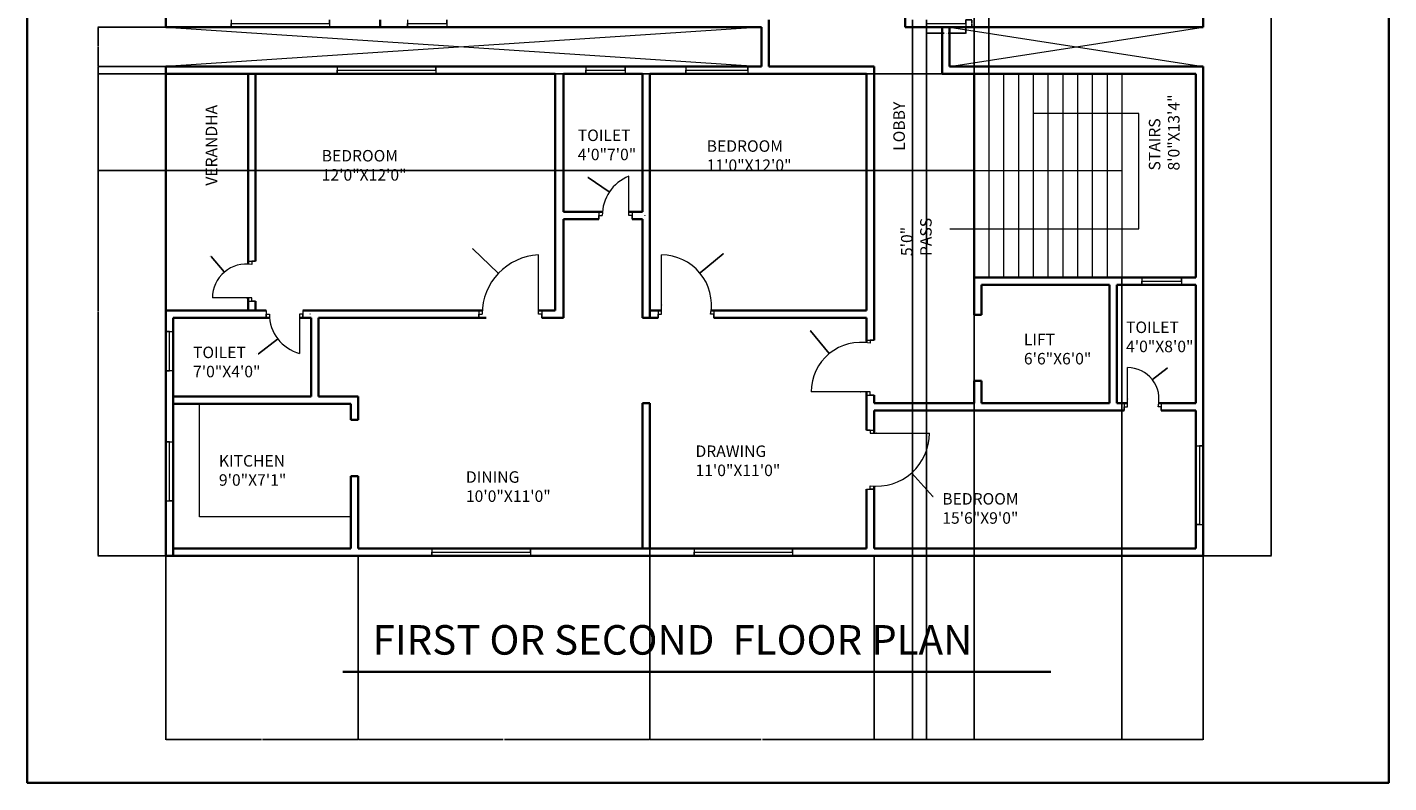
# Model space of a CAD drawing. Units: inches. Extents: x 6393 to 7221, y 6416 to 7347.
# Tile 1 of 3: x 6393 to 7221, y 6416 to 6876. Entities that reach past the tile are written whole.
import ezdxf

# ---------------------------------------------------------------- set-up
doc = ezdxf.new("R2010")
doc.units = ezdxf.units.IN
for name, color, linetype, lineweight in [('A-ANNO-DIMS', 2, 'Continuous', 18), ('A-ANNO-TEXT', 7, 'Continuous', 35), ('A-ANNO-TTLB', 7, 'Continuous', 35), ('A-AREA-IDEN', 7, 'Continuous', 18), ('A-DOOR', 3, 'Continuous', 18), ('A-FLOR-FIXT', 8, 'Continuous', 18), ('A-FLOR-OPEN', 8, 'Continuous', 13), ('A-FLOR-STRS', 7, 'Continuous', 18), ('A-GLAZ', 4, 'Continuous', 18), ('A-WALL', 7, 'Continuous', 35)]:
    doc.layers.add(name, color=color, linetype=linetype, lineweight=lineweight)
doc.styles.get("Standard").update_dxf_attribs({"font": 'arial.ttf'})
doc.dimstyles.get("Standard").update_dxf_attribs({"dimtxt": 0.18, "dimasz": 0.18, "dimexe": 0.18, "dimexo": 0.0625, "dimgap": 0.09, "dimtad": 0, "dimtih": 1, "dimtoh": 1, "dimdec": 4, "dimzin": 0, "dimdsep": 46, "dimtxsty": 'Standard', "dimcen": 0.09, "dimadec": 0, "dimazin": 0, "dimtfac": 1, "dimtdec": 4, "dimtofl": 0, "dimtmove": 0, "dimatfit": 3, "dimfxl": 1, "dimtolj": 1, "dimtzin": 0, "dimarcsym": 0})

# ---------------------------------------------------------------- blocks, each defined once
blk = doc.blocks.new('WIN-60IN')
for p, q in [((0, 60), (4.5, 60)), ((4.5, 60), (2.25, 60)), ((2.25, 60), (2.25, 0)), ((2.25, 0), (0, 0)), ((0, 0), (4.5, 0))]:
    blk.add_line(p, q)
blk = doc.blocks.new('WIN-24IN')
for p, q in [((0, 4.5), (0, 0)), ((0, 0), (0, 2.25)), ((0, 2.25), (24, 2.25)), ((24, 2.25), (24, 4.5)), ((24, 4.5), (24, 0))]:
    blk.add_line(p, q)
blk = doc.blocks.new('WIN-48IN')
for p, q in [((0, 4.5), (0, 0)), ((0, 0), (0, 2.25)), ((0, 2.25), (48, 2.25)), ((48, 2.25), (48, 4.5)), ((48, 4.5), (48, 0))]:
    blk.add_line(p, q)
blk = doc.blocks.new('*D7')
at = {"layer": 'A-ANNO-DIMS', "color": 0, "lineweight": -2, "transparency": 16777216}
for p, q in [((6939.9, 6876.26), (6939.9, 6872.55)), ((6940.08, 6872.73), (6950.67, 6872.73)), ((6963.72, 6872.73), (6953.14, 6872.73)), ((6963.9, 6876.26), (6963.9, 6872.55))]:
    blk.add_line(p, q, dxfattribs=at)
at = {"layer": 'A-ANNO-DIMS', "color": 0, "transparency": 16777216}
for points in [[(6940.08, 6872.76), (6940.08, 6872.7), (6939.9, 6872.73)], [(6963.72, 6872.76), (6963.72, 6872.7), (6963.9, 6872.73)]]:
    blk.add_solid(points, dxfattribs=at)
at = {"layer": 'Defpoints', "color": 0, "transparency": 16777216}
for p in [(6939.9, 6876.33), (6963.9, 6876.33), (6963.9, 6872.73)]:
    blk.add_point(p, dxfattribs=at)
at = {"layer": 'A-ANNO-DIMS', "color": 0, "transparency": 16777216, "insert": (6951.9, 6872.73), "char_height": 0.18, "attachment_point": 5}
blk.add_mtext('\\A1;WINDOW B 24 TYP.', dxfattribs=at)
blk = doc.blocks.new('*D8')
at = {"layer": 'A-ANNO-DIMS', "color": 0, "lineweight": -2, "transparency": 16777216}
for p, q in [((6963.97, 6880.83), (6967.68, 6880.83)), ((6967.5, 6880.65), (6967.5, 6878.76)), ((6963.97, 6876.33), (6967.68, 6876.33)), ((6967.5, 6876.51), (6967.5, 6878.4))]:
    blk.add_line(p, q, dxfattribs=at)
at = {"layer": 'A-ANNO-DIMS', "color": 0, "transparency": 16777216}
for points in [[(6967.47, 6880.65), (6967.53, 6880.65), (6967.5, 6880.83)], [(6967.47, 6876.51), (6967.53, 6876.51), (6967.5, 6876.33)]]:
    blk.add_solid(points, dxfattribs=at)
at = {"layer": 'Defpoints', "color": 0, "transparency": 16777216}
for p in [(6963.9, 6880.83), (6967.5, 6880.83), (6963.9, 6876.33)]:
    blk.add_point(p, dxfattribs=at)
at = {"layer": 'A-ANNO-DIMS', "color": 0, "transparency": 16777216, "insert": (6967.5, 6878.58), "char_height": 0.18, "attachment_point": 5}
blk.add_mtext('\\A1;5 TYP.', dxfattribs=at)
blk = doc.blocks.new('*D14')
at = {"layer": 'A-ANNO-DIMS', "color": 0, "lineweight": -2, "transparency": 16777216}
for p, q in [((7108.59, 7305.82), (7149.96, 7305.82)), ((7149.78, 7305.64), (7149.78, 6930.26)), ((7149.78, 6554.51), (7149.78, 6929.89)), ((7108.49, 6554.33), (7149.96, 6554.33))]:
    blk.add_line(p, q, dxfattribs=at)
at = {"layer": 'A-ANNO-DIMS', "color": 0, "transparency": 16777216}
for points in [[(7149.75, 7305.64), (7149.81, 7305.64), (7149.78, 7305.82)], [(7149.75, 6554.51), (7149.81, 6554.51), (7149.78, 6554.33)]]:
    blk.add_solid(points, dxfattribs=at)
at = {"layer": 'Defpoints', "color": 0, "transparency": 16777216}
for p in [(7108.53, 7305.82), (7149.78, 7305.82), (7108.43, 6554.33)]:
    blk.add_point(p, dxfattribs=at)
at = {"layer": 'A-ANNO-DIMS', "color": 0, "transparency": 16777216, "insert": (7149.78, 6930.07), "char_height": 0.18, "attachment_point": 5}
blk.add_mtext('\\A1;751.5', dxfattribs=at)
blk = doc.blocks.new('*D15')
at = {"layer": 'A-ANNO-DIMS', "color": 0, "lineweight": -2, "transparency": 16777216}
for p, q in [((6476.86, 6852.33), (6435.5, 6852.33)), ((6435.68, 6852.15), (6435.68, 6703.51)), ((6435.68, 6554.51), (6435.68, 6703.14)), ((6476.86, 6554.33), (6435.5, 6554.33))]:
    blk.add_line(p, q, dxfattribs=at)
at = {"layer": 'A-ANNO-DIMS', "color": 0, "transparency": 16777216}
for points in [[(6435.65, 6852.15), (6435.71, 6852.15), (6435.68, 6852.33)], [(6435.65, 6554.51), (6435.71, 6554.51), (6435.68, 6554.33)]]:
    blk.add_solid(points, dxfattribs=at)
at = {"layer": 'Defpoints', "color": 0, "transparency": 16777216}
for p in [(6435.68, 6852.33), (6476.93, 6852.33), (6476.93, 6554.33)]:
    blk.add_point(p, dxfattribs=at)
at = {"layer": 'A-ANNO-DIMS', "color": 0, "transparency": 16777216, "insert": (6435.68, 6703.33), "char_height": 0.18, "attachment_point": 5}
blk.add_mtext('\\A1;298', dxfattribs=at)
blk = doc.blocks.new('*D16')
at = {"layer": 'A-ANNO-DIMS', "color": 0, "lineweight": -2, "transparency": 16777216}
for p, q in [((6476.86, 6876.33), (6435.5, 6876.33)), ((6435.68, 6876.15), (6435.68, 6864.51)), ((6435.68, 6852.51), (6435.68, 6864.15)), ((6476.86, 6852.33), (6435.5, 6852.33))]:
    blk.add_line(p, q, dxfattribs=at)
at = {"layer": 'A-ANNO-DIMS', "color": 0, "transparency": 16777216}
for points in [[(6435.65, 6876.15), (6435.71, 6876.15), (6435.68, 6876.33)], [(6435.65, 6852.51), (6435.71, 6852.51), (6435.68, 6852.33)]]:
    blk.add_solid(points, dxfattribs=at)
at = {"layer": 'Defpoints', "color": 0, "transparency": 16777216}
for p in [(6435.68, 6876.33), (6476.93, 6876.33), (6476.93, 6852.33)]:
    blk.add_point(p, dxfattribs=at)
at = {"layer": 'A-ANNO-DIMS', "color": 0, "transparency": 16777216, "insert": (6435.68, 6864.33), "char_height": 0.18, "attachment_point": 5}
blk.add_mtext('\\A1;24', dxfattribs=at)
blk = doc.blocks.new('*D22')
at = {"layer": 'A-ANNO-DIMS', "color": 0, "lineweight": -2, "transparency": 16777216}
for p, q in [((6476.93, 6554.26), (6476.93, 6442.29)), ((6593.93, 6554.26), (6593.93, 6442.29)), ((6477.11, 6442.47), (6535.15, 6442.47)), ((6593.75, 6442.47), (6535.71, 6442.47))]:
    blk.add_line(p, q, dxfattribs=at)
at = {"layer": 'A-ANNO-DIMS', "color": 0, "transparency": 16777216}
for points in [[(6477.11, 6442.5), (6477.11, 6442.44), (6476.93, 6442.47)], [(6593.75, 6442.5), (6593.75, 6442.44), (6593.93, 6442.47)]]:
    blk.add_solid(points, dxfattribs=at)
at = {"layer": 'Defpoints', "color": 0, "transparency": 16777216}
for p in [(6476.93, 6554.33), (6593.93, 6554.33), (6593.93, 6442.47)]:
    blk.add_point(p, dxfattribs=at)
at = {"layer": 'A-ANNO-DIMS', "color": 0, "transparency": 16777216, "insert": (6535.43, 6442.47), "char_height": 0.18, "attachment_point": 5}
blk.add_mtext('\\A1;117', dxfattribs=at)
blk = doc.blocks.new('*D23')
at = {"layer": 'A-ANNO-DIMS', "color": 0, "lineweight": -2, "transparency": 16777216}
for p, q in [((6771.53, 6558.76), (6771.53, 6442.29)), ((6593.93, 6554.26), (6593.93, 6442.29)), ((6594.11, 6442.47), (6682.34, 6442.47)), ((6771.35, 6442.47), (6683.12, 6442.47))]:
    blk.add_line(p, q, dxfattribs=at)
at = {"layer": 'A-ANNO-DIMS', "color": 0, "transparency": 16777216}
for points in [[(6594.11, 6442.5), (6594.11, 6442.44), (6593.93, 6442.47)], [(6771.35, 6442.5), (6771.35, 6442.44), (6771.53, 6442.47)]]:
    blk.add_solid(points, dxfattribs=at)
at = {"layer": 'Defpoints', "color": 0, "transparency": 16777216}
for p in [(6771.53, 6558.83), (6593.93, 6554.33), (6771.53, 6442.47)]:
    blk.add_point(p, dxfattribs=at)
at = {"layer": 'A-ANNO-DIMS', "color": 0, "transparency": 16777216, "insert": (6682.73, 6442.47), "char_height": 0.18, "attachment_point": 5}
blk.add_mtext('\\A1;177.6', dxfattribs=at)
blk = doc.blocks.new('*D24')
at = {"layer": 'A-ANNO-DIMS', "color": 0, "lineweight": -2, "transparency": 16777216}
for p, q in [((6771.53, 6558.76), (6771.53, 6442.29)), ((6908.03, 6554.26), (6908.03, 6442.29)), ((6771.71, 6442.47), (6839.4, 6442.47)), ((6907.85, 6442.47), (6840.17, 6442.47))]:
    blk.add_line(p, q, dxfattribs=at)
at = {"layer": 'A-ANNO-DIMS', "color": 0, "transparency": 16777216}
for points in [[(6771.71, 6442.5), (6771.71, 6442.44), (6771.53, 6442.47)], [(6907.85, 6442.5), (6907.85, 6442.44), (6908.03, 6442.47)]]:
    blk.add_solid(points, dxfattribs=at)
at = {"layer": 'Defpoints', "color": 0, "transparency": 16777216}
for p in [(6771.53, 6558.83), (6908.03, 6554.33), (6908.03, 6442.47)]:
    blk.add_point(p, dxfattribs=at)
at = {"layer": 'A-ANNO-DIMS', "color": 0, "transparency": 16777216, "insert": (6839.78, 6442.47), "char_height": 0.18, "attachment_point": 5}
blk.add_mtext('\\A1;136.5', dxfattribs=at)
blk = doc.blocks.new('*D25')
at = {"layer": 'A-ANNO-DIMS', "color": 0, "lineweight": -2, "transparency": 16777216}
for p, q in [((6908.03, 6554.26), (6908.03, 6442.29)), ((7108.43, 6554.26), (7108.43, 6442.29)), ((6908.21, 6442.47), (7007.84, 6442.47)), ((7108.25, 6442.47), (7008.62, 6442.47))]:
    blk.add_line(p, q, dxfattribs=at)
at = {"layer": 'A-ANNO-DIMS', "color": 0, "transparency": 16777216}
for points in [[(6908.21, 6442.5), (6908.21, 6442.44), (6908.03, 6442.47)], [(7108.25, 6442.5), (7108.25, 6442.44), (7108.43, 6442.47)]]:
    blk.add_solid(points, dxfattribs=at)
at = {"layer": 'Defpoints', "color": 0, "transparency": 16777216}
for p in [(6908.03, 6554.33), (7108.43, 6554.33), (7108.43, 6442.47)]:
    blk.add_point(p, dxfattribs=at)
at = {"layer": 'A-ANNO-DIMS', "color": 0, "transparency": 16777216, "insert": (7008.23, 6442.47), "char_height": 0.18, "attachment_point": 5}
blk.add_mtext('\\A1;200.4', dxfattribs=at)
blk = doc.blocks.new('*D29')
at = {"layer": 'A-ANNO-DIMS', "color": 0, "lineweight": -2, "transparency": 16777216}
for p, q in [((6968.93, 6847.89), (6968.93, 7347.25)), ((6969.11, 7347.07), (6973.28, 7347.07)), ((6977.75, 7347.07), (6973.58, 7347.07)), ((6977.93, 6847.89), (6977.93, 7347.25))]:
    blk.add_line(p, q, dxfattribs=at)
at = {"layer": 'A-ANNO-DIMS', "color": 0, "transparency": 16777216}
for points in [[(6969.11, 7347.1), (6969.11, 7347.04), (6968.93, 7347.07)], [(6977.75, 7347.1), (6977.75, 7347.04), (6977.93, 7347.07)]]:
    blk.add_solid(points, dxfattribs=at)
at = {"layer": 'Defpoints', "color": 0, "transparency": 16777216}
for p in [(6977.93, 7347.07), (6968.93, 6847.83), (6977.93, 6847.83)]:
    blk.add_point(p, dxfattribs=at)
at = {"layer": 'A-ANNO-DIMS', "color": 0, "transparency": 16777216, "insert": (6973.43, 7347.07), "char_height": 0.18, "attachment_point": 5}
blk.add_mtext('\\A1;9', dxfattribs=at)
blk = doc.blocks.new('*D30')
at = {"layer": 'A-ANNO-DIMS', "color": 0, "lineweight": -2, "transparency": 16777216}
for p, q in [((6968.93, 6723.75), (6968.93, 6442.29)), ((7058.93, 6723.75), (7058.93, 6442.29)), ((6969.11, 6442.47), (7013.71, 6442.47)), ((7058.75, 6442.47), (7014.15, 6442.47))]:
    blk.add_line(p, q, dxfattribs=at)
at = {"layer": 'A-ANNO-DIMS', "color": 0, "transparency": 16777216}
for points in [[(6969.11, 6442.5), (6969.11, 6442.44), (6968.93, 6442.47)], [(7058.75, 6442.5), (7058.75, 6442.44), (7058.93, 6442.47)]]:
    blk.add_solid(points, dxfattribs=at)
at = {"layer": 'Defpoints', "color": 0, "transparency": 16777216}
for p in [(6968.93, 6723.82), (7058.93, 6723.82), (7058.93, 6442.47)]:
    blk.add_point(p, dxfattribs=at)
at = {"layer": 'A-ANNO-DIMS', "color": 0, "transparency": 16777216, "insert": (7013.93, 6442.47), "char_height": 0.18, "attachment_point": 5}
blk.add_mtext('\\A1;90', dxfattribs=at)
blk = doc.blocks.new('*D31')
at = {"layer": 'A-ANNO-DIMS', "color": 0, "lineweight": -2, "transparency": 16777216}
for p, q in [((6968.86, 6847.83), (6435.5, 6847.83)), ((6435.68, 6847.65), (6435.68, 6818.65)), ((6435.68, 6789.28), (6435.68, 6818.28)), ((6968.86, 6789.1), (6435.5, 6789.1))]:
    blk.add_line(p, q, dxfattribs=at)
at = {"layer": 'A-ANNO-DIMS', "color": 0, "transparency": 16777216}
for points in [[(6435.65, 6847.65), (6435.71, 6847.65), (6435.68, 6847.83)], [(6435.65, 6789.28), (6435.71, 6789.28), (6435.68, 6789.1)]]:
    blk.add_solid(points, dxfattribs=at)
at = {"layer": 'Defpoints', "color": 0, "transparency": 16777216}
for p in [(6435.68, 6847.83), (6968.93, 6847.83), (6968.93, 6789.1)]:
    blk.add_point(p, dxfattribs=at)
at = {"layer": 'A-ANNO-DIMS', "color": 0, "transparency": 16777216, "insert": (6435.68, 6818.46), "char_height": 0.18, "attachment_point": 5}
blk.add_mtext('\\A1;58.73', dxfattribs=at)
blk = doc.blocks.new('*D32')
at = {"layer": 'A-ANNO-DIMS', "color": 0, "lineweight": -2, "transparency": 16777216}
for p, q in [((6931.43, 6880.76), (6931.43, 6442.29)), ((6939.9, 6880.76), (6939.9, 6442.29)), ((6931.61, 6442.47), (6935.27, 6442.47)), ((6939.72, 6442.47), (6936.06, 6442.47))]:
    blk.add_line(p, q, dxfattribs=at)
at = {"layer": 'A-ANNO-DIMS', "color": 0, "transparency": 16777216}
for points in [[(6931.61, 6442.5), (6931.61, 6442.44), (6931.43, 6442.47)], [(6939.72, 6442.5), (6939.72, 6442.44), (6939.9, 6442.47)]]:
    blk.add_solid(points, dxfattribs=at)
at = {"layer": 'Defpoints', "color": 0, "transparency": 16777216}
for p in [(6931.43, 6880.83), (6939.9, 6880.83), (6939.9, 6442.47)]:
    blk.add_point(p, dxfattribs=at)
at = {"layer": 'A-ANNO-DIMS', "color": 0, "transparency": 16777216, "insert": (6935.67, 6442.47), "char_height": 0.18, "attachment_point": 5}
blk.add_mtext('\\A1;8.477', dxfattribs=at)
blk = doc.blocks.new('*D37')
at = {"layer": 'A-ANNO-DIMS', "color": 0, "lineweight": -2, "transparency": 16777216}
for p, q in [((6663.56, 6741.37), (6663.74, 6741.37)), ((6663.74, 6741.37), (6679.26, 6726.57)), ((6705.38, 6701.58), (6705.56, 6701.58)), ((6705.47, 6701.49), (6705.47, 6701.67))]:
    blk.add_line(p, q, dxfattribs=at)
at = {"layer": 'A-ANNO-DIMS', "color": 0, "transparency": 16777216}
blk.add_solid([(6679.28, 6726.6), (6679.24, 6726.55), (6679.39, 6726.45)], dxfattribs=at)
at = {"layer": 'Defpoints', "color": 0, "transparency": 16777216}
for p in [(6679.39, 6726.45), (6705.47, 6701.58)]:
    blk.add_point(p, dxfattribs=at)
at = {"layer": 'A-ANNO-DIMS', "color": 0, "transparency": 16777216, "insert": (6663.08, 6741.37), "char_height": 0.18, "attachment_point": 5}
blk.add_mtext('\\A1;R36.04', dxfattribs=at)
blk = doc.blocks.new('*D38')
at = {"layer": 'A-ANNO-DIMS', "color": 0, "lineweight": -2, "transparency": 16777216}
for p, q in [((6909.47, 6628.94), (6909.65, 6628.94)), ((6909.56, 6628.85), (6909.56, 6629.03)), ((6943.81, 6590.4), (6931.09, 6604.72)), ((6943.99, 6590.4), (6943.81, 6590.4))]:
    blk.add_line(p, q, dxfattribs=at)
at = {"layer": 'A-ANNO-DIMS', "color": 0, "transparency": 16777216}
blk.add_solid([(6931.11, 6604.74), (6931.07, 6604.7), (6930.97, 6604.85)], dxfattribs=at)
at = {"layer": 'Defpoints', "color": 0, "transparency": 16777216}
for p in [(6909.56, 6628.94), (6930.97, 6604.85)]:
    blk.add_point(p, dxfattribs=at)
at = {"layer": 'A-ANNO-DIMS', "color": 0, "transparency": 16777216, "insert": (6944.47, 6590.4), "char_height": 0.18, "attachment_point": 5}
blk.add_mtext('\\A1;R32.22', dxfattribs=at)
blk = doc.blocks.new('*D41')
at = {"layer": 'A-ANNO-DIMS', "color": 0, "lineweight": -2, "transparency": 16777216}
for p, q in [((6816.12, 6738.24), (6802.23, 6726.71)), ((6816.3, 6738.24), (6816.12, 6738.24)), ((6778.61, 6707.18), (6778.79, 6707.18)), ((6778.7, 6707.09), (6778.7, 6707.27))]:
    blk.add_line(p, q, dxfattribs=at)
at = {"layer": 'A-ANNO-DIMS', "color": 0, "transparency": 16777216}
blk.add_solid([(6802.21, 6726.73), (6802.24, 6726.68), (6802.09, 6726.59)], dxfattribs=at)
at = {"layer": 'Defpoints', "color": 0, "transparency": 16777216}
for p in [(6802.09, 6726.59), (6778.7, 6707.18)]:
    blk.add_point(p, dxfattribs=at)
at = {"layer": 'A-ANNO-DIMS', "color": 0, "transparency": 16777216, "insert": (6816.71, 6738.24), "char_height": 0.18, "attachment_point": 5}
blk.add_mtext('\\A1;R30.4', dxfattribs=at)
blk = doc.blocks.new('*D43')
at = {"layer": 'A-ANNO-DIMS', "color": 0, "lineweight": -2, "transparency": 16777216}
for p, q in [((6869.13, 6691.47), (6869.31, 6691.47)), ((6869.31, 6691.47), (6880.68, 6677.63)), ((6899.84, 6654.2), (6900.02, 6654.2)), ((6899.93, 6654.11), (6899.93, 6654.29))]:
    blk.add_line(p, q, dxfattribs=at)
at = {"layer": 'A-ANNO-DIMS', "color": 0, "transparency": 16777216}
blk.add_solid([(6880.7, 6677.65), (6880.66, 6677.61), (6880.79, 6677.49)], dxfattribs=at)
at = {"layer": 'Defpoints', "color": 0, "transparency": 16777216}
for p in [(6880.79, 6677.49), (6899.93, 6654.2)]:
    blk.add_point(p, dxfattribs=at)
at = {"layer": 'A-ANNO-DIMS', "color": 0, "transparency": 16777216, "insert": (6868.58, 6691.47), "char_height": 0.18, "attachment_point": 5}
blk.add_mtext('\\A1;R30.144', dxfattribs=at)
blk = doc.blocks.new('*D48')
at = {"layer": 'A-ANNO-DIMS', "color": 0, "lineweight": -2, "transparency": 16777216}
for p, q in [((6733.9, 6784.71), (6734.08, 6784.71)), ((6734.08, 6784.71), (6746.84, 6776.13)), ((6768.42, 6761.58), (6768.6, 6761.58)), ((6768.51, 6761.49), (6768.51, 6761.67))]:
    blk.add_line(p, q, dxfattribs=at)
at = {"layer": 'A-ANNO-DIMS', "color": 0, "transparency": 16777216}
blk.add_solid([(6746.86, 6776.16), (6746.82, 6776.11), (6746.99, 6776.03)], dxfattribs=at)
at = {"layer": 'Defpoints', "color": 0, "transparency": 16777216}
for p in [(6746.99, 6776.03), (6768.51, 6761.58)]:
    blk.add_point(p, dxfattribs=at)
at = {"layer": 'A-ANNO-DIMS', "color": 0, "transparency": 16777216, "insert": (6733.42, 6784.71), "char_height": 0.18, "attachment_point": 5}
blk.add_mtext('\\A1;R25.92', dxfattribs=at)
blk = doc.blocks.new('*D50')
at = {"layer": 'A-ANNO-DIMS', "color": 0, "lineweight": -2, "transparency": 16777216}
for p, q in [((6564.67, 6701.58), (6564.85, 6701.58)), ((6564.76, 6701.49), (6564.76, 6701.67)), ((6533.25, 6677.36), (6544.92, 6686.33)), ((6533.07, 6677.36), (6533.25, 6677.36))]:
    blk.add_line(p, q, dxfattribs=at)
at = {"layer": 'A-ANNO-DIMS', "color": 0, "transparency": 16777216}
blk.add_solid([(6544.9, 6686.36), (6544.94, 6686.31), (6545.06, 6686.44)], dxfattribs=at)
at = {"layer": 'Defpoints', "color": 0, "transparency": 16777216}
for p in [(6564.76, 6701.58), (6545.06, 6686.44)]:
    blk.add_point(p, dxfattribs=at)
at = {"layer": 'A-ANNO-DIMS', "color": 0, "transparency": 16777216, "insert": (6532.59, 6677.36), "char_height": 0.18, "attachment_point": 5}
blk.add_mtext('\\A1;R24.84', dxfattribs=at)
blk = doc.blocks.new('*D52')
at = {"layer": 'A-ANNO-DIMS', "color": 0, "lineweight": -2, "transparency": 16777216}
for p, q in [((6504.37, 6736.59), (6504.55, 6736.59)), ((6504.55, 6736.59), (6512.42, 6727.3)), ((6525.75, 6711.44), (6525.93, 6711.44)), ((6525.84, 6711.35), (6525.84, 6711.53))]:
    blk.add_line(p, q, dxfattribs=at)
at = {"layer": 'A-ANNO-DIMS', "color": 0, "transparency": 16777216}
blk.add_solid([(6512.44, 6727.31), (6512.39, 6727.28), (6512.53, 6727.16)], dxfattribs=at)
at = {"layer": 'Defpoints', "color": 0, "transparency": 16777216}
for p in [(6512.53, 6727.16), (6525.84, 6711.44)]:
    blk.add_point(p, dxfattribs=at)
at = {"layer": 'A-ANNO-DIMS', "color": 0, "transparency": 16777216, "insert": (6503.96, 6736.59), "char_height": 0.18, "attachment_point": 5}
blk.add_mtext('\\A1;R20.6', dxfattribs=at)
blk = doc.blocks.new('*D54')
at = {"layer": 'A-ANNO-DIMS', "color": 0, "lineweight": -2, "transparency": 16777216}
for p, q in [((7086.59, 6668.66), (7077.64, 6661.7)), ((7086.77, 6668.66), (7086.59, 6668.66)), ((7062.25, 6649.81), (7062.43, 6649.81)), ((7062.34, 6649.72), (7062.34, 6649.9))]:
    blk.add_line(p, q, dxfattribs=at)
at = {"layer": 'A-ANNO-DIMS', "color": 0, "transparency": 16777216}
blk.add_solid([(7077.62, 6661.72), (7077.66, 6661.68), (7077.5, 6661.59)], dxfattribs=at)
at = {"layer": 'Defpoints', "color": 0, "transparency": 16777216}
for p in [(7077.5, 6661.59), (7062.34, 6649.81)]:
    blk.add_point(p, dxfattribs=at)
at = {"layer": 'A-ANNO-DIMS', "color": 0, "transparency": 16777216, "insert": (7087.32, 6668.66), "char_height": 0.18, "attachment_point": 5}
blk.add_mtext('\\A1;R19.196', dxfattribs=at)

msp = doc.modelspace()

# ---------------------------------------------------------------- linework, layer by layer
at = {"layer": 'A-ANNO-TEXT'}
msp.add_line((6584.6832, 6483.7206), (7015.6392, 6483.7206), dxfattribs=at)
at = {"layer": 'A-ANNO-TTLB'}
msp.add_lwpolyline([(6392.5039, 7327.0003), (7221.4173, 7327.0003), (7221.4173, 6416.0496), (6392.5039, 6416.0496)], close=True, dxfattribs=at)
at = {"layer": 'A-DOOR'}
for p, q in [((6758.7113, 6761.5767), (6758.7113, 6785.5767)), ((6740.5842, 6763.8267), (6740.5842, 6759.3267)), ((6740.5842, 6759.3267), (6740.5842, 6761.5767)), ((6740.5842, 6761.5767), (6742.5842, 6761.5767)), ((6760.7113, 6761.5767), (6758.7113, 6761.5767)), ((6760.7113, 6763.8267), (6760.7113, 6759.3267)), ((6760.7113, 6759.3267), (6760.7113, 6761.5767)), ((6526.9926, 6733.7527), (6531.4926, 6733.7527)), ((6531.4926, 6733.7527), (6529.2426, 6733.7527)), ((6529.2426, 6733.7527), (6529.2426, 6731.7527)), ((6703.7607, 6701.5767), (6703.7607, 6737.5767)), ((6778.6963, 6701.5767), (6778.6963, 6737.5767)), ((6529.2426, 6711.4356), (6505.2426, 6711.4356)), ((6526.9926, 6709.4356), (6531.4926, 6709.4356)), ((6529.2426, 6709.4356), (6529.2426, 6711.4356)), ((6531.4926, 6709.4356), (6529.2426, 6709.4356)), ((6537.9203, 6703.8267), (6537.9203, 6699.3267)), ((6537.9203, 6699.3267), (6537.9203, 6701.5767)), ((6537.9203, 6701.5767), (6539.9203, 6701.5767)), ((6560.3619, 6701.5767), (6558.3619, 6701.5767)), ((6558.3619, 6701.5767), (6558.3619, 6677.5767)), ((6560.3619, 6703.8267), (6560.3619, 6699.3267)), ((6560.3619, 6699.3267), (6560.3619, 6701.5767)), ((6667.4273, 6703.8267), (6667.4273, 6699.3267)), ((6667.4273, 6699.3267), (6667.4273, 6701.5767)), ((6667.4273, 6701.5767), (6669.4273, 6701.5767)), ((6705.7607, 6701.5767), (6703.7607, 6701.5767)), ((6705.7607, 6703.8267), (6705.7607, 6699.3267)), ((6705.7607, 6699.3267), (6705.7607, 6701.5767)), ((6776.6963, 6703.8267), (6776.6963, 6699.3267)), ((6776.6963, 6699.3267), (6776.6963, 6701.5767)), ((6776.6963, 6701.5767), (6778.6963, 6701.5767)), ((6810.5725, 6701.5767), (6808.5725, 6701.5767)), ((6810.5725, 6703.8267), (6810.5725, 6699.3267)), ((6810.5725, 6699.3267), (6810.5725, 6701.5767)), ((6903.5328, 6685.7708), (6908.0328, 6685.7708)), ((6908.0328, 6685.7708), (6905.7828, 6685.7708)), ((6905.7828, 6685.7708), (6905.7828, 6683.7708)), ((7062.3379, 6645.0112), (7062.3379, 6669.0112)), ((6905.7828, 6654.2006), (6869.7828, 6654.2006)), ((6903.5328, 6652.2006), (6908.0328, 6652.2006)), ((6905.7828, 6652.2006), (6905.7828, 6654.2006)), ((6908.0328, 6652.2006), (6905.7828, 6652.2006)), ((7060.3379, 6647.3153), (7060.3379, 6644.2968)), ((7060.3379, 6642.8153), (7060.3379, 6645.0112)), ((7060.3379, 6645.0112), (7062.3379, 6645.0112)), ((7060.3379, 6644.2968), (7060.3379, 6642.8153)), ((7082.9373, 6645.0653), (7080.9373, 6645.0653)), ((7082.9373, 6647.3153), (7082.9373, 6642.8153)), ((7082.9373, 6642.8153), (7082.9373, 6645.0653)), ((6905.7828, 6630.9369), (6903.5328, 6630.9369)), ((6903.5328, 6630.9369), (6908.0328, 6630.9369)), ((6905.7828, 6630.9369), (6905.7828, 6628.9369)), ((6905.7828, 6628.9369), (6929.7828, 6628.9369)), ((6929.7828, 6628.9369), (6941.7828, 6628.9369)), ((6903.5328, 6594.9369), (6908.0328, 6594.9369)), ((6905.7828, 6594.9369), (6905.7828, 6596.9369)), ((6908.0328, 6594.9369), (6905.7828, 6594.9369))]:
    msp.add_line(p, q, dxfattribs=at)
for centre, radius, start, end in [((6768.5058, 6761.5767), 25.9217, 112.2006208, 180), ((6525.8422, 6711.4356), 20.5997, 80.4988436, 180), ((6705.4677, 6701.5767), 36.0405, 92.7148426, 180), ((6778.6963, 6707.1797), 30.397, 349.3781844, 90), ((6564.758, 6701.5767), 24.8377, 180, 255.0772597), ((6899.9272, 6654.2006), 30.1444, 78.7990306, 180), ((7062.3379, 6649.8148), 19.1963, 345.6751584, 90), ((6909.5605, 6628.9369), 32.2222, 263.2670787, 0)]:
    msp.add_arc(centre, radius, start, end, dxfattribs=at)
at = {"layer": 'A-FLOR-FIXT'}
for p, q in [((6497.2871, 6578.0115), (6497.2871, 6646.8267)), ((6589.4273, 6578.0115), (6497.2871, 6578.0115))]:
    msp.add_line(p, q, dxfattribs=at)
at = {"layer": 'A-FLOR-OPEN'}
for p, q in [((6839.4675, 6876.3267), (6476.9273, 6852.3267)), ((6476.9273, 6876.3267), (6839.4675, 6852.3267)), ((6953.9273, 6852.3267), (7108.4273, 6876.3267)), ((6953.9273, 6876.3267), (7108.4273, 6852.3267))]:
    msp.add_line(p, q, dxfattribs=at)
at = {"layer": 'A-FLOR-STRS'}
for p, q in [((6977.9273, 6847.8267), (6977.9273, 6723.8153)), ((6986.9273, 6847.8267), (6986.9273, 6723.8153)), ((6995.9273, 6847.8267), (6995.9273, 6723.8153)), ((7004.9273, 6847.8267), (7004.9273, 6723.8153)), ((7013.9273, 6847.8267), (7013.9273, 6723.8153)), ((7022.9273, 6847.8267), (7022.9273, 6723.8153)), ((7031.9273, 6847.8267), (7031.9273, 6723.8153)), ((7040.9273, 6847.8267), (7040.9273, 6723.8153)), ((7049.9273, 6847.8267), (7049.9273, 6723.8153)), ((7058.9273, 6847.8267), (7058.9273, 6723.8153)), ((7069.2754, 6823.7446), (7004.9273, 6823.7446)), ((7069.2754, 6753.5578), (7069.2754, 6823.7446)), ((6968.9273, 6789.1013), (7058.9273, 6789.1013)), ((6954.1119, 6753.5578), (7069.2754, 6753.5578))]:
    msp.add_line(p, q, dxfattribs=at)
at = {"layer": 'A-GLAZ'}
for p, q in [((6793.4269, 6852.3267), (6793.4269, 6847.8267)), ((6793.4269, 6847.8267), (6793.4269, 6850.0767)), ((6793.4269, 6850.0767), (6831.3061, 6850.0767)), ((6831.3061, 6850.0767), (6831.3061, 6852.3267)), ((6831.3061, 6852.3267), (6831.3061, 6847.8267)), ((6479.1773, 6691.0447), (6476.9273, 6691.0447)), ((6476.9273, 6691.0447), (6481.4273, 6691.0447)), ((6479.1773, 6667.0447), (6479.1773, 6691.0447)), ((6481.4273, 6667.0447), (6476.9273, 6667.0447)), ((6476.9273, 6667.0447), (6479.1773, 6667.0447)), ((6479.1773, 6623.8458), (6476.9273, 6623.8458)), ((6476.9273, 6623.8458), (6481.4273, 6623.8458)), ((6479.1773, 6587.8458), (6479.1773, 6623.8458)), ((6476.9273, 6587.8458), (6481.4273, 6587.8458)), ((6481.4273, 6587.8458), (6479.1773, 6587.8458)), ((6638.8994, 6554.3267), (6638.8994, 6554.3267))]:
    msp.add_line(p, q, dxfattribs=at)
at = {"layer": 'A-WALL'}
for p, q in [((6476.9273, 7254.3267), (6476.9273, 6876.3267)), ((7108.4273, 7254.3267), (7108.4273, 6876.3267)), ((6926.9273, 6969.3267), (6926.9273, 6876.3267)), ((6607.4273, 6880.8267), (6607.4273, 6876.3267)), ((6843.9675, 6852.3267), (6843.9675, 6880.8267)), ((6476.9273, 6876.3267), (6839.4675, 6876.3267)), ((6839.4675, 6876.3267), (6839.4675, 6852.3267)), ((6843.9675, 6876.3267), (6843.9675, 6852.3267)), ((6931.4273, 6876.3267), (6926.9273, 6876.3267)), ((6926.9273, 6876.3267), (7103.9273, 6876.3267)), ((6953.9273, 6876.3267), (6949.4273, 6876.3267)), ((6949.4273, 6876.3267), (6949.4273, 6852.3267)), ((6953.9273, 6876.3267), (6953.9273, 6852.3267)), ((7103.9273, 6876.3267), (7108.4273, 6876.3267)), ((6476.9273, 6852.3267), (6839.4675, 6852.3267)), ((6476.9273, 6852.3267), (6476.9273, 6554.3267)), ((6481.4273, 6847.8267), (6476.9273, 6847.8267)), ((6481.4273, 6847.8267), (6653.9273, 6847.8267)), ((6526.9926, 6847.8267), (6526.9926, 6740.9824)), ((6531.4926, 6740.9824), (6531.4926, 6847.8267)), ((6611.9273, 6847.8267), (6713.9273, 6847.8267)), ((6713.9273, 6847.8267), (6713.9273, 6703.8267)), ((6719.0328, 6847.8267), (6719.0328, 6763.8267)), ((6719.0328, 6847.8267), (6719.0328, 6763.8267)), ((6719.0328, 6847.8267), (6719.0328, 6763.8267)), ((6719.0328, 6847.8267), (6767.0328, 6847.8267)), ((6767.0328, 6847.8267), (6767.0328, 6763.8267)), ((6771.5328, 6847.8267), (6771.5328, 6703.8267)), ((6771.5328, 6847.8267), (6903.5328, 6847.8267)), ((6843.9675, 6852.3267), (6908.0328, 6852.3267)), ((6903.5328, 6847.8267), (6903.5328, 6703.8267)), ((6908.0328, 6847.8267), (6908.0328, 6852.3267)), ((6908.0328, 6847.8267), (6908.0328, 6699.3267)), ((6908.0328, 6847.8267), (6908.0328, 6699.3267)), ((6949.4273, 6852.3267), (6949.4273, 6847.8267)), ((6949.4273, 6847.8267), (7103.9273, 6847.8267)), ((6953.9273, 6852.3267), (7103.9273, 6852.3267)), ((6968.9273, 6847.8267), (6968.9273, 6701.0574)), ((7103.9273, 6852.3267), (7108.4273, 6852.3267)), ((7103.9273, 6847.8267), (7103.9273, 6723.8153)), ((7108.4273, 6852.3267), (7108.4273, 6554.3267)), ((6719.0328, 6763.8267), (6742.682, 6763.8267)), ((6740.5842, 6759.3267), (6719.0328, 6759.3267)), ((6719.0328, 6759.3267), (6719.0328, 6699.3267)), ((6719.0328, 6759.3267), (6719.0328, 6699.3267)), ((6758.7113, 6763.8267), (6767.0328, 6763.8267)), ((6767.0328, 6759.3267), (6760.7113, 6759.3267)), ((6767.0328, 6759.3267), (6767.0328, 6699.3267)), ((6526.9926, 6740.9824), (6526.9926, 6732.0031)), ((6531.4926, 6733.7527), (6531.4926, 6740.9824)), ((6968.9273, 6723.8153), (7103.9273, 6723.8153)), ((6973.4273, 6719.3153), (7051.4273, 6719.3153)), ((6973.4273, 6719.3153), (6973.4273, 6701.0574)), ((7051.4273, 6719.3153), (7051.4273, 6647.3153)), ((7055.9273, 6719.3153), (7055.9273, 6647.3153)), ((7055.9273, 6719.3153), (7103.9273, 6719.3153)), ((7103.9273, 6719.3153), (7103.9273, 6647.3153)), ((6526.9926, 6711.4356), (6526.9926, 6703.8267)), ((6531.4926, 6703.8267), (6531.4926, 6709.4356)), ((6476.9273, 6703.8267), (6476.9273, 6699.3267)), ((6481.4273, 6703.8267), (6476.9273, 6703.8267)), ((6537.9203, 6703.8267), (6481.4273, 6703.8267)), ((6481.4273, 6699.3267), (6540.0224, 6699.3267)), ((6481.4273, 6699.3267), (6481.4273, 6554.3267)), ((6526.9926, 6703.8267), (6531.4926, 6703.8267)), ((6558.3619, 6699.3267), (6565.4273, 6699.3267)), ((6667.4273, 6703.8267), (6560.3619, 6703.8267)), ((6565.4273, 6703.8267), (6569.9273, 6703.8267)), ((6565.4273, 6651.3267), (6565.4273, 6699.3267)), ((6569.9273, 6699.3267), (6569.9273, 6651.3267)), ((6569.9273, 6699.3267), (6667.4273, 6699.3267)), ((6667.4273, 6703.8267), (6669.4976, 6703.8267)), ((6667.4273, 6699.3267), (6671.9273, 6699.3267)), ((6703.7607, 6703.8267), (6713.9273, 6703.8267)), ((6705.7607, 6699.3267), (6719.0328, 6699.3267)), ((6714.771, 6699.3267), (6719.0328, 6699.3267)), ((6767.0328, 6699.3267), (6776.6963, 6699.3267)), ((6778.6963, 6703.8267), (6771.5328, 6703.8267)), ((6771.5328, 6703.8267), (6771.5328, 6699.3267)), ((6903.5328, 6703.8267), (6808.9079, 6703.8267)), ((6810.5725, 6699.3267), (6903.5328, 6699.3267)), ((6903.5328, 6684.1286), (6903.5328, 6699.3267)), ((6908.0328, 6699.3267), (6908.0328, 6703.8267)), ((6908.0328, 6701.5767), (6908.0328, 6699.3267)), ((6908.0328, 6699.3267), (6908.0328, 6685.7708)), ((6968.9273, 6701.0574), (6973.4273, 6701.0574)), ((6968.9273, 6660.9028), (6973.4273, 6660.9028)), ((6968.9273, 6660.9028), (6968.9273, 6647.3153)), ((6973.4273, 6660.9028), (6973.4273, 6647.3153)), ((6481.4273, 6651.3267), (6565.4273, 6651.3267)), ((6481.4273, 6651.3267), (6565.4273, 6651.3267)), ((6569.9273, 6651.3267), (6593.9273, 6651.3267)), ((6593.9273, 6637.1004), (6593.9273, 6651.3267)), ((6903.5328, 6647.3153), (6903.5328, 6654.2006)), ((6908.0328, 6652.2006), (6908.0328, 6647.3153)), ((6481.4273, 6646.8267), (6589.4273, 6646.8267)), ((6481.4273, 6646.8267), (6589.4273, 6646.8267)), ((6589.4273, 6646.8267), (6589.4273, 6637.1004)), ((6767.0328, 6647.3153), (6767.0328, 6558.8267)), ((6767.0328, 6647.3153), (6771.5328, 6647.3153)), ((6771.5328, 6647.3153), (6771.5328, 6558.8267)), ((6903.5328, 6647.3153), (6903.5328, 6647.3153)), ((6903.5328, 6630.9369), (6903.5328, 6647.3153)), ((6968.0328, 6647.3153), (6908.0328, 6647.3153)), ((6908.0328, 6647.3153), (6915.5261, 6647.3153)), ((6908.0328, 6642.8153), (6908.0328, 6628.9369)), ((6908.0328, 6642.8153), (6968.0328, 6642.8153)), ((6915.5261, 6642.8153), (6908.0328, 6642.8153)), ((6968.0328, 6647.3153), (6968.9273, 6647.3153)), ((7060.3379, 6642.8153), (6968.0328, 6642.8153)), ((6973.4273, 6647.3153), (7051.4273, 6647.3153)), ((7055.9273, 6647.3153), (7062.3379, 6647.3153)), ((7081.3708, 6647.3153), (7103.9273, 6647.3153)), ((7103.9273, 6642.8153), (7082.9373, 6642.8153)), ((7103.9273, 6642.8153), (7103.9273, 6558.8267)), ((6589.4273, 6637.1004), (6593.9273, 6637.1004)), ((6593.9273, 6602.8267), (6589.4273, 6602.8267)), ((6589.4273, 6602.8267), (6589.4273, 6558.8267)), ((6593.9273, 6558.8267), (6593.9273, 6602.8267)), ((6903.5328, 6558.8267), (6903.5328, 6594.9369)), ((6908.0328, 6596.7509), (6908.0328, 6558.8267)), ((6481.4273, 6558.8267), (6589.4273, 6558.8267)), ((6593.9273, 6558.8267), (6903.5328, 6558.8267)), ((6908.0328, 6558.8267), (7046.2962, 6558.8267)), ((7103.9273, 6558.8267), (7046.2962, 6558.8267)), ((7108.4273, 6554.3267), (7108.4273, 6558.8267)), ((6476.9273, 6554.3267), (6593.9273, 6554.3267)), ((6589.4273, 6554.3267), (6593.9273, 6554.3267)), ((6593.9273, 6554.3267), (6908.0328, 6554.3267)), ((6908.0328, 6554.3267), (6903.5328, 6554.3267)), ((6905.7828, 6554.3267), (6974.0723, 6554.3267)), ((7046.2962, 6554.3267), (6974.0723, 6554.3267)), ((7046.2962, 6554.3267), (7108.4273, 6554.3267))]:
    msp.add_line(p, q, dxfattribs=at)

# ---------------------------------------------------------------- block references
at = {"layer": 'A-GLAZ', "extrusion": (0, 0, -1), "zscale": -1, "rotation": 270}
for name, p in [('WIN-60IN', (-6576.5769, 6880.827)), ('WIN-60IN', (-6641.2312, 6852.327)), ('WIN-48IN', (-7108.427, 6621.3729)), ('WIN-60IN', (-6698.8997, 6558.827)), ('WIN-60IN', (-6858.4377, 6558.827))]:
    msp.add_blockref(name, p, dxfattribs=at)
at = {"layer": 'A-GLAZ'}
for p in [(6623.9861, 6876.327), (6939.905, 6876.327), (6732.5155, 6847.827), (7071.1634, 6719.3156)]:
    msp.add_blockref('WIN-24IN', p, dxfattribs=at)

# ---------------------------------------------------------------- texts
at = {"layer": 'A-ANNO-TEXT', "insert": (6602.7271, 6512.1019), "char_height": 18, "attachment_point": 1}
msp.add_mtext_dynamic_manual_height_columns('FIRST OR SECOND  FLOOR PLAN', width=498.617319, gutter_width=12.5, heights=[0], dxfattribs=at)
at = {"layer": 'A-AREA-IDEN', "char_height": 7, "attachment_point": 1, "rotation": 90}
for s, width, insert in [('LOBBY', 51.838069, (6919.8019, 6801.019)), ('STAIRS\\P8\'0"X13\'4"', 57.279963, (7075.3514, 6789.0295)), ('VERANDHA', 109.767921, (6501.1556, 6779.7974)), ('5\'0" PASS', 26.261269, (6924.4638, 6736.9128))]:
    msp.add_mtext_dynamic_manual_height_columns(s, width=width, gutter_width=12.5, heights=[0], dxfattribs=dict(at, insert=insert))
at = {"layer": 'A-AREA-IDEN', "char_height": 7, "attachment_point": 1}
for s, width, insert in [('TOILET\\P4\'0"7\'0"', 43.84626, (6727.6865, 6813.9759)), ('BEDROOM\\P11\'0"X12\'0"', 88.342356, (6806.1669, 6807.4325)), ('BEDROOM\\P12\'0"X12\'0"', 75.188021, (6571.7888, 6801.5298)), ('LIFT\\P6\'6"X6\'0"', 39.580469, (6999.2858, 6689.577)), ('TOILET\\P4\'0"X8\'0"', 50.252532, (7061.4776, 6697.0336)), ('TOILET\\P7\'0"X4\'0"', 51.579396, (6493.4559, 6681.7353)), ('KITCHEN\\P9\'0"X7\'1"', 100.486104, (6509.1978, 6615.6661)), ('DRAWING\\P11\'0"X11\'0"', 69.065089, (6799.3475, 6621.5292)), ('DINING\\P10\'0"X11\'0"', 62.14176, (6659.5765, 6605.8204)), ('BEDROOM\\P15\'6"X9\'0"', 80.086023, (6949.5938, 6592.5219))]:
    msp.add_mtext_dynamic_manual_height_columns(s, width=width, gutter_width=12.5, heights=[0], dxfattribs=dict(at, insert=insert))

# ---------------------------------------------------------------- dimensions: what is measured, and where the dimension line sits
at = {"layer": 'A-ANNO-DIMS'}
for base, p1, p2, override, picture, middle in [((6977.9273, 7347.0726), (6968.9273, 6847.8267), (6977.9273, 6847.8267), {"dimdec": 0, "dimlfac": 1, "dimrnd": 0, "dimzin": 0, "dimdsep": 46, "dimlunit": 2}, '*D29', (6973.4273, 7347.0726)), ((6939.9047, 6442.4706), (6931.4273, 6880.8267), (6939.9047, 6880.8267), {"dimdec": 3, "dimlfac": 1, "dimrnd": 0, "dimzin": 0, "dimdsep": 46, "dimlunit": 2}, '*D32', (6935.666, 6442.4706)), ((7058.9273, 6442.4706), (6968.9273, 6723.8153), (7058.9273, 6723.8153), {"dimdec": 0, "dimlfac": 1, "dimrnd": 0, "dimzin": 0, "dimdsep": 46, "dimlunit": 2}, '*D30', (7013.9273, 6442.4706)), ((6771.5328, 6442.4706), (6593.9273, 6554.3267), (6771.5328, 6558.8267), {"dimdec": 1, "dimlfac": 1, "dimrnd": 0, "dimzin": 0, "dimdsep": 46, "dimlunit": 2}, '*D23', (6682.73, 6442.4706)), ((6908.0328, 6442.4706), (6771.5328, 6558.8267), (6908.0328, 6554.3267), {"dimdec": 1, "dimlfac": 1, "dimrnd": 0, "dimzin": 0, "dimdsep": 46, "dimlunit": 2}, '*D24', (6839.7828, 6442.4706)), ((6593.9273, 6442.4706), (6476.9273, 6554.3267), (6593.9273, 6554.3267), {"dimdec": 0, "dimlfac": 1, "dimrnd": 0, "dimzin": 0, "dimdsep": 46, "dimlunit": 2}, '*D22', (6535.4273, 6442.4706)), ((7108.4273, 6442.4706), (6908.0328, 6554.3267), (7108.4273, 6554.3267), {"dimdec": 1, "dimlfac": 1, "dimrnd": 0, "dimzin": 0, "dimdsep": 46, "dimlunit": 2}, '*D25', (7008.23, 6442.4706))]:
    dim = msp.add_linear_dim(base=base, p1=p1, p2=p2, dimstyle='Standard', override=override, dxfattribs=at)
    dim.commit()
    dim.dimension.update_dxf_attribs({"geometry": picture, "text_midpoint": middle})
for base, p1, p2, override, picture, middle in [((7149.7774, 7305.8226), (7108.4273, 6554.3267), (7108.5274, 7305.8226), {"dimdec": 1, "dimlfac": 1, "dimrnd": 0, "dimzin": 0, "dimdsep": 46, "dimlunit": 2}, '*D14', (7149.7774, 6930.0747)), ((6435.6773, 6876.3267), (6476.9273, 6852.3267), (6476.9273, 6876.3267), {"dimdec": 0, "dimlfac": 1, "dimrnd": 0, "dimzin": 0, "dimdsep": 46, "dimlunit": 2}, '*D16', (6435.6773, 6864.3267)), ((6435.6773, 6847.8267), (6968.9273, 6789.1013), (6968.9273, 6847.8267), {"dimdec": 2, "dimlfac": 1, "dimrnd": 0, "dimzin": 0, "dimdsep": 46, "dimlunit": 2}, '*D31', (6435.6773, 6818.464)), ((6435.6773, 6852.3267), (6476.9273, 6554.3267), (6476.9273, 6852.3267), {"dimdec": 0, "dimlfac": 1, "dimrnd": 0, "dimzin": 0, "dimdsep": 46, "dimlunit": 2}, '*D15', (6435.6773, 6703.3267))]:
    dim = msp.add_linear_dim(base=base, p1=p1, p2=p2, angle=90, dimstyle='Standard', override=override, dxfattribs=at)
    dim.commit()
    dim.dimension.update_dxf_attribs({"geometry": picture, "text_midpoint": middle})
dim = msp.add_linear_dim(base=(6967.5047315606, 6880.8267298921), p1=(6963.9047315606, 6876.3267298921), p2=(6963.9047315606, 6880.8267298921), angle=90, text='<> TYP.', dimstyle='Standard', override={"dimdec": 0, "dimlfac": 1, "dimrnd": 0, "dimzin": 0, "dimdsep": 46, "dimlunit": 2}, dxfattribs=at)
dim.commit()
dim.dimension.update_dxf_attribs({"geometry": '*D8', "text_midpoint": (6967.5047315606, 6878.5767298921)})
dim = msp.add_linear_dim(base=(6963.9047, 6872.7267), p1=(6939.9047, 6876.3267), p2=(6963.9047, 6876.3267), text='WINDOW B <> TYP.', dimstyle='Standard', override={"dimdec": 0, "dimlfac": 1, "dimrnd": 0, "dimzin": 0, "dimdsep": 46, "dimlunit": 2}, dxfattribs=at)
dim.commit()
dim.dimension.update_dxf_attribs({"geometry": '*D7', "text_midpoint": (6951.9047, 6872.7267)})
for center, mpoint, override, picture, middle in [((6768.5058, 6761.5767), (6746.9902, 6776.0339), {"dimdec": 2, "dimlfac": 1, "dimrnd": 0, "dimzin": 0, "dimdsep": 46, "dimlunit": 2}, '*D48', (6733.4219, 6784.7082)), ((6705.4677, 6701.5767), (6679.3867, 6726.4503), {"dimdec": 2, "dimlfac": 1, "dimrnd": 0, "dimzin": 0, "dimdsep": 46, "dimlunit": 2}, '*D37', (6663.0786, 6741.3744)), ((6525.8422, 6711.4356), (6512.5322, 6727.1578), {"dimdec": 1, "dimlfac": 1, "dimrnd": 0, "dimzin": 0, "dimdsep": 46, "dimlunit": 2}, '*D52', (6503.9563, 6736.5911)), ((6778.6963, 6707.1797), (6802.0872, 6726.5922), {"dimdec": 1, "dimlfac": 1, "dimrnd": 0, "dimzin": 0, "dimdsep": 46, "dimlunit": 2}, '*D41', (6816.7113, 6738.2397)), ((6564.758, 6701.5767), (6545.0632, 6686.4432), {"dimdec": 2, "dimlfac": 1, "dimrnd": 0, "dimzin": 0, "dimdsep": 46, "dimlunit": 2}, '*D50', (6532.5869, 6677.363)), ((6899.9272, 6654.2006), (6880.7938, 6677.4943), {"dimdec": 3, "dimlfac": 1, "dimrnd": 0, "dimzin": 0, "dimdsep": 46, "dimlunit": 2}, '*D43', (6868.5843, 6691.4705)), ((7062.3379, 6649.8148), (7077.4983, 6661.5902), {"dimdec": 3, "dimlfac": 1, "dimrnd": 0, "dimzin": 0, "dimdsep": 46, "dimlunit": 2}, '*D54', (7087.3243, 6668.6555)), ((6909.5605, 6628.9369), (6930.9681, 6604.8539), {"dimdec": 2, "dimlfac": 1, "dimrnd": 0, "dimzin": 0, "dimdsep": 46, "dimlunit": 2}, '*D38', (6944.4715, 6590.4041))]:
    dim = msp.add_radius_dim(center=center, mpoint=mpoint, dimstyle='Standard', override=override, dxfattribs=at)
    dim.commit()
    dim.dimension.update_dxf_attribs({"geometry": picture, "text_midpoint": middle, "dimtype": 164})

doc.saveas('drawing.dxf')
